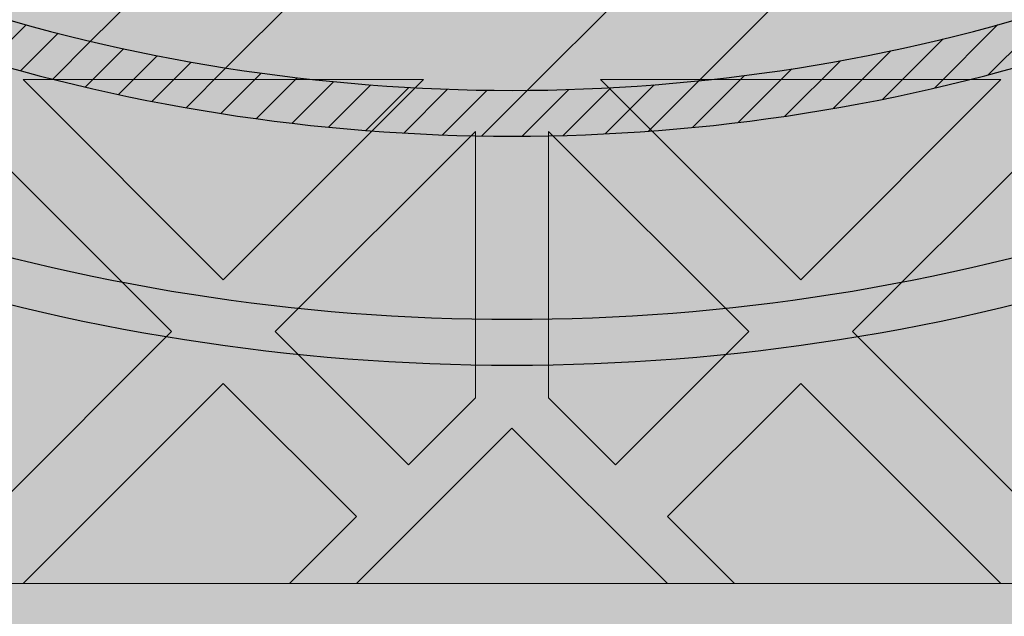
# Model space of a CAD drawing. Units: inches. Extents: x 844 to 2234, y 346 to 1084.
# Tile 10 of 93: x 1121.143 to 1124.57, y 686.542 to 688.619. Entities that reach past the tile are written whole.
import ezdxf

# ---------------------------------------------------------------- set-up
doc = ezdxf.new("R2010")
doc.units = ezdxf.units.IN
doc.header["$MEASUREMENT"] = 0
for name, color, linetype, lineweight in [('A-ANNO-DIMS', 2, 'Continuous', 18), ('furniture', 8, 'Continuous', 18), ('RA-AP-01$0$INT', 35, 'Continuous', 5)]:
    doc.layers.add(name, color=color, linetype=linetype, lineweight=lineweight)
doc.layers.add('RA-AP-01$0$FURN', color=3, linetype='Continuous')
doc.layers.add('RA-AP-01$0$WOOD', color=64, linetype='Continuous')
doc.styles.get("Standard").update_dxf_attribs({"font": 'arial.ttf'})
doc.dimstyles.get("Standard").update_dxf_attribs({"dimtxt": 6, "dimasz": 3, "dimexe": 0.18, "dimexo": 0.0625, "dimgap": 0.09, "dimtad": 0, "dimtih": 1, "dimtoh": 1, "dimdec": 1, "dimzin": 0, "dimdsep": 46, "dimlunit": 3, "dimtxsty": 'Standard', "dimblk": 'ARCHTICK', "dimcen": 0.09, "dimadec": 0, "dimazin": 0, "dimtfac": 1, "dimtdec": 1, "dimtofl": 0, "dimtmove": 0, "dimatfit": 3, "dimfxl": 1, "dimtolj": 1, "dimtzin": 0, "dimarcsym": 0})

# ---------------------------------------------------------------- blocks, each defined once
blk = doc.blocks.new('A$C18D01794')
at = {"layer": 'RA-AP-01$0$INT'}
blk.add_hatch(color=256, dxfattribs=at).paths.add_polyline_path([(4.505206456958071, -6.306712009588038), (5.305206456958072, -6.306712009588038), (5.305206456958072, -7.106712009588038), (5.255206456951893, -7.10671200958804), (5.25520645694868, -6.356712009605972), (4.555206456959269, -6.356712009587461), (4.555206456956052, -7.106712009588038), (4.505206456958073, -7.106712009588038)])
h = blk.add_hatch(color=256, dxfattribs=at)
h.paths.add_polyline_path([(4.585917135068448, -6.356712009588273), (4.614201406330596, -6.356712009589021), (4.668846067270487, -6.411356670531338), (4.723490728212344, -6.356712009591912), (4.771774999457151, -6.35671200959319), (4.826419660396886, -6.411356670535356), (4.862780050090322, -6.374996280843536), (4.844495778842715, -6.356712009595112), (4.862780050090411, -6.356712009595595), (4.905206456960182, -6.399138416468211), (4.947632863832445, -6.356712009597838), (4.965917135079675, -6.356712009598322), (4.947632863831759, -6.374996280845421), (4.983993253523576, -6.411356670538857), (5.038637914464627, -6.356712009600247), (5.08692218571208, -6.356712009601523), (5.141566846649976, -6.411356670541852), (5.196211507589851, -6.356712009604411), (5.224495778822615, -6.356712009605161), (4.905206456953975, -6.676001331473793)])
h.paths.add_polyline_path([(4.895206456956031, -6.637717060225675), (4.895206456958921, -6.528427738347902), (4.840561796018589, -6.583072399285802)], flags=16)
h.paths.add_polyline_path([(4.915206456955638, -6.637717060226121), (4.969851117895509, -6.583072399288678), (4.915206456957609, -6.528427738348344)], flags=16)
h.paths.add_polyline_path([(4.826419660395175, -6.568930263661755), (4.881064321335613, -6.514285602723745), (4.771774999456703, -6.514285602720857)], flags=16)
h.paths.add_polyline_path([(4.983993253519558, -6.568930263665262), (5.038637914460456, -6.514285602726792), (4.929348592581548, -6.514285602724816)], flags=16)
h.paths.add_polyline_path([(4.881064321336025, -6.494285602723742), (4.826419660397532, -6.439640941782821), (4.771774999457062, -6.494285602720859)], flags=16)
h.paths.add_polyline_path([(4.929348592582019, -6.494285602724817), (5.038637914460982, -6.494285602726792), (4.983993253522945, -6.439640941786327)], flags=16)
h.paths.add_polyline_path([(4.895206456960191, -6.480143467100443), (4.895206456962115, -6.407422687715913), (4.876922185715016, -6.389138416467584), (4.840561796021581, -6.425498806159401)], flags=16)
h.paths.add_polyline_path([(4.915206456958487, -6.480143467100889), (4.969851117899527, -6.425498806162279), (4.933490728206909, -6.389138416468043), (4.9152064569598, -6.40742268771434)], flags=16)
h.paths.add_polyline_path([(4.757632863832376, -6.480143467096812), (4.812277524772842, -6.425498806158772), (4.757632863834348, -6.370854145217844)], flags=16)
h.paths.add_polyline_path([(4.737632863832376, -6.480143467096286), (4.737632863834348, -6.370854145217375), (4.682988202893906, -6.425498806155385)], flags=16)
h.paths.add_polyline_path([(5.05278005008503, -6.480143467103376), (5.052780050087917, -6.370854145224413), (4.998135389146995, -6.425498806162908)], flags=16)
h.paths.add_polyline_path([(5.072780050085024, -6.480143467103744), (5.127424711025931, -6.42549880616527), (5.072780050087916, -6.370854145224832)], flags=16)
h.paths.add_polyline_path([(4.935917135072783, -6.706712009592292), (5.255206456948811, -6.387422687716309), (5.255206456948932, -6.415706958964177), (5.200561796010279, -6.470351619902839), (5.255206456949403, -6.524996280841948), (5.25520645694961, -6.5732805520894), (5.200561796009787, -6.627925213029239), (5.236922185702417, -6.664285602721864), (5.255206456949919, -6.646001331474357), (5.255206456949998, -6.664285602721898), (5.212780050078687, -6.706712009592262), (5.25520645695036, -6.749138416463932), (5.255206456950438, -6.767422687711313), (5.236922185702424, -6.749138416463297), (5.200561796009796, -6.785498806155928), (5.255206456950753, -6.840143467096874), (5.25520645695096, -6.888427738341682), (5.200561796010322, -6.943072399282328), (5.255206456951428, -6.997717060223427), (5.255206456951547, -7.026001331471006)])
h.paths.add_polyline_path([(5.042988202883395, -6.785498806155427), (5.097632863823085, -6.840143467095101), (5.097632863822622, -6.730854145216193)], flags=16)
h.paths.add_polyline_path([(5.028846067259663, -6.771356670531693), (5.083490728198774, -6.716712009592573), (4.974201406321001, -6.716712009593042)], flags=16)
h.paths.add_polyline_path([(5.117632863823087, -6.840143467095186), (5.172277524762331, -6.785498806155926), (5.11763286382262, -6.730854145216225)], flags=16)
h.paths.add_polyline_path([(5.08349072819877, -6.696712009593886), (5.028846067259652, -6.642067348654775), (4.974201406320998, -6.696712009593438)], flags=16)
h.paths.add_polyline_path([(5.131774999446817, -6.854285602718917), (5.186419660386065, -6.799640941779662), (5.241064321325782, -6.854285602719365)], flags=17)
h.paths.add_polyline_path([(5.131774999446228, -6.716712009592374), (5.186419660386065, -6.771356670532194), (5.222780050079488, -6.734996280838764), (5.204495778832781, -6.716712009592063)], flags=16)
h.paths.add_polyline_path([(5.097632863822613, -6.682569873970264), (5.097632863823061, -6.573280552091354), (5.042988202883383, -6.627925213031044)], flags=16)
h.paths.add_polyline_path([(5.131774999446899, -6.874285602718915), (5.241064321325809, -6.874285602719364), (5.186419660386591, -6.928930263658598)], flags=17)
h.paths.add_polyline_path([(5.131774999446226, -6.696712009594078), (5.204495778830767, -6.696712009594374), (5.22278005007868, -6.67842773834687), (5.186419660386049, -6.642067348654249)], flags=16)
h.paths.add_polyline_path([(5.11763286382262, -6.682569873970225), (5.17227752476232, -6.627925213030515), (5.117632863823064, -6.573280552091267)], flags=16)
h.paths.add_polyline_path([(5.186419660386069, -6.613783077405491), (5.241064321325754, -6.559138416465795), (5.131774999446791, -6.559138416466263)], flags=16)
h.paths.add_polyline_path([(5.131774999446872, -6.539138416466263), (5.24106432132578, -6.539138416465794), (5.186419660386554, -6.484493755526573)], flags=16)
h.paths.add_polyline_path([(5.255206456951811, -7.08742268770861), (5.255206456951895, -7.106712009588038), (4.555206456956052, -7.106712009588038), (4.555206456956136, -7.087422687708617), (4.905206456953973, -6.737422687710788)])
h.paths.add_polyline_path([(4.983993253513404, -6.8444937555241), (4.92934859257295, -6.899138416462108), (5.03863791445186, -6.899138416465014)], flags=16)
h.paths.add_polyline_path([(4.969851117889988, -6.83035161990006), (4.915206456952556, -6.775706958960171), (4.915206456949648, -6.884996280837944)], flags=16)
h.paths.add_polyline_path([(4.929348592572535, -6.919138416462105), (4.983993253511019, -6.973783077403037), (5.038637914451496, -6.919138416465012)], flags=16)
h.paths.add_polyline_path([(5.052780050074912, -6.93328055208906), (4.998135389134438, -6.987925213027088), (5.052780050072919, -7.042569873968025)], flags=16)
h.paths.add_polyline_path([(5.07278005007491, -6.933280552089588), (5.072780050072918, -7.042569873968497), (5.127424711013374, -6.987925213030498)], flags=16)
h.paths.add_polyline_path([(4.89520645695295, -6.775706958959721), (4.840561796013067, -6.830351619897157), (4.895206456950961, -6.884996280837494)], flags=16)
h.paths.add_polyline_path([(4.915206456948365, -6.933280552085403), (4.915206456946434, -7.006001331471951), (4.933490728192729, -7.024285602719066), (4.969851117886972, -6.987925213026453)], flags=16)
h.paths.add_polyline_path([(4.881064321327021, -6.899138416461022), (4.82641966038902, -6.84449375552057), (4.771774999448108, -6.899138416459029)], flags=16)
h.paths.add_polyline_path([(4.895206456950073, -6.933280552084951), (4.840561796009022, -6.987925213023558), (4.876922185700835, -7.024285602716997), (4.895206456948749, -7.006001331469487)], flags=16)
h.paths.add_polyline_path([(4.983993253510392, -7.0020673486505), (4.947632863816944, -7.038427738342319), (4.965917135064043, -7.05671200959023), (5.038637914448995, -7.056712009591555)], flags=16)
h.paths.add_polyline_path([(4.881064321326543, -6.91913841646102), (4.771774999447578, -6.919138416459031), (4.826419660385607, -6.973783077399508)], flags=16)
h.paths.add_polyline_path([(4.905206456946447, -7.014285602717636), (4.862780050074785, -7.056712009588352), (4.947632863816685, -7.056712009589775)], flags=16)
h.paths.add_polyline_path([(5.14156684663679, -7.002067348654549), (5.086922185696452, -7.056712009592438), (5.196211507574223, -7.056712009594425)], flags=16)
h.paths.add_polyline_path([(4.8264196603837, -7.002067348646972), (4.771774999442643, -7.056712009585575), (4.8444957788276, -7.056712009587508), (4.862780050075511, -7.038427738340416)], flags=16)
h.paths.add_polyline_path([(4.812277524760289, -6.98792521302292), (4.757632863822258, -6.933280552082447), (4.757632863819352, -7.042569873961408)], flags=16)
h.paths.add_polyline_path([(4.73763286382226, -6.933280552082079), (4.682988202881349, -6.987925213020536), (4.737632863819352, -7.04256987396099)], flags=16)
h.paths.add_polyline_path([(4.723490728195188, -7.056712009584289), (4.668846067257299, -7.002067348643949), (4.614201406317417, -7.056712009581383)], flags=16)
h.paths.add_polyline_path([(4.597632863829262, -6.706712009592262), (4.555206456957951, -6.664285602721896), (4.555206456958029, -6.646001331474357), (4.573490728205535, -6.664285602721864), (4.609851117898167, -6.627925213029238), (4.555206456958338, -6.573280552089402), (4.555206456958546, -6.524996280841952), (4.60985111789767, -6.470351619902839), (4.555206456959015, -6.415706958964177), (4.555206456959138, -6.387422687716309), (4.874495778835167, -6.70671200959229), (4.5552064569564, -7.026001331471015), (4.555206456956523, -6.997717060223433), (4.609851117897629, -6.94307239928233), (4.555206456956988, -6.888427738341681), (4.555206456957198, -6.840143467096881), (4.609851117898153, -6.78549880615593), (4.573490728205528, -6.749138416463297), (4.555206456957507, -6.76742268771132), (4.555206456957585, -6.749138416463933)])
h.paths.add_polyline_path([(4.712780050085332, -6.730854145216195), (4.712780050084863, -6.840143467095105), (4.767424711024555, -6.785498806155427)], flags=16)
h.paths.add_polyline_path([(4.726922185709173, -6.716712009592573), (4.781566846648288, -6.771356670531693), (4.836211507586949, -6.716712009593043)], flags=16)
h.paths.add_polyline_path([(4.692780050085327, -6.730854145216225), (4.638135389145619, -6.785498806155928), (4.692780050084865, -6.840143467095185)], flags=16)
h.paths.add_polyline_path([(4.726922185709182, -6.696712009593886), (4.836211507586949, -6.696712009593436), (4.7815668466483, -6.642067348654773)], flags=16)
h.paths.add_polyline_path([(4.678637914461726, -6.71671200959237), (4.605917135075169, -6.716712009592063), (4.587632863828464, -6.734996280838766), (4.623993253521887, -6.771356670532195)], flags=16)
h.paths.add_polyline_path([(4.712780050085336, -6.68256987397026), (4.767424711024568, -6.627925213031042), (4.71278005008489, -6.573280552091352)], flags=16)
h.paths.add_polyline_path([(4.678637914461726, -6.696712009594076), (4.623993253521899, -6.642067348654247), (4.587632863829271, -6.67842773834687), (4.605917135077185, -6.696712009594376)], flags=16)
h.paths.add_polyline_path([(4.692780050085336, -6.682569873970228), (4.692780050084889, -6.573280552091267), (4.638135389145632, -6.627925213030515)], flags=16)
h.paths.add_polyline_path([(4.623993253521885, -6.799640941779662), (4.678637914461131, -6.854285602718915), (4.56934859258217, -6.854285602719365)], flags=17)
h.paths.add_polyline_path([(4.623993253521901, -6.613783077405509), (4.678637914461158, -6.559138416466263), (4.569348592582195, -6.559138416465795)], flags=16)
h.paths.add_polyline_path([(4.678637914461051, -6.874285602718915), (4.623993253521361, -6.928930263658598), (4.569348592582143, -6.874285602719364)], flags=17)
h.paths.add_polyline_path([(4.678637914461076, -6.539138416466263), (4.623993253521399, -6.484493755526573), (4.569348592582167, -6.539138416465796)], flags=16)
h = blk.add_hatch(color=256, dxfattribs=at)
h.paths.add_polyline_path([(4.969851117891331, -6.583072399286455), (4.915206456952669, -6.63771706022511), (4.915206456952222, -6.528427738347337)])
h.paths.add_polyline_path([(4.895206456953064, -6.637717060225108), (4.840561796014413, -6.583072399286448), (4.895206456953533, -6.528427738347335)])
h.paths.add_polyline_path([(4.826419660390684, -6.568930263662714), (4.771774999451003, -6.514285602723024), (4.881064321329913, -6.514285602723489)])
h.paths.add_polyline_path([(4.881064321329884, -6.494285602723492), (4.771774999450921, -6.494285602723024), (4.82641966039018, -6.439640941783778)])
h.paths.add_polyline_path([(4.895206456953734, -6.48014346709988), (4.840561796013912, -6.425498806160046), (4.876922185707337, -6.389138416466622), (4.895206456954043, -6.40742268771333)])
h.paths.add_polyline_path([(4.862780050082808, -6.374996280843689), (4.826419660390178, -6.411356670536314), (4.771774999450351, -6.356712009596481), (4.844495778835303, -6.356712009596181)])
h.paths.add_polyline_path([(4.812277524766446, -6.425498806160041), (4.757632863827191, -6.480143467099289), (4.757632863826741, -6.370854145220329)])
h.paths.add_polyline_path([(4.737632863827191, -6.480143467099214), (4.682988202887508, -6.425498806159518), (4.737632863826743, -6.370854145220299)])
h.paths.add_polyline_path([(4.668846067263777, -6.41135667053579), (4.614201406325123, -6.356712009597128), (4.723490728202894, -6.356712009596675)])
h.paths.add_polyline_path([(4.905206456953846, -6.399138416467422), (4.862780050082654, -6.356712009596229), (4.947632863824561, -6.356712009595756)])
h.paths.add_polyline_path([(4.915206456952028, -6.480143467099882), (4.91520645695173, -6.407422687715346), (4.933490728199234, -6.389138416467428), (4.96985111789186, -6.425498806160055)])
h.paths.add_polyline_path([(5.038637914454841, -6.494285602723048), (4.929348592575874, -6.494285602723497), (4.983993253515593, -6.439640941783787)])
h.paths.add_polyline_path([(4.983993253515065, -6.568930263662725), (4.929348592575849, -6.514285602723495), (5.038637914454755, -6.514285602723045)])
h.paths.add_polyline_path([(5.052780050079843, -6.480143467099317), (4.998135389140595, -6.425498806160058), (5.052780050080309, -6.370854145220356)])
h.paths.add_polyline_path([(4.983993253516868, -6.411356670536324), (4.947632863824241, -6.374996280843694), (4.965917135071747, -6.356712009596188), (5.038637914456701, -6.356712009596504)])
h.paths.add_polyline_path([(5.127424711019533, -6.425498806159557), (5.072780050079843, -6.480143467099239), (5.07278005008031, -6.370854145220326)])
h.paths.add_polyline_path([(5.141566846643269, -6.411356670535829), (5.086922185704154, -6.356712009596707), (5.196211507581929, -6.356712009597176)])
for p, q in [((4.555206456959269, -6.356712009587461), (5.255206456948681, -6.356712009605972)), ((4.771774999458274, -6.356712009594314), (4.826419660396887, -6.411356670535356)), ((4.844495778843225, -6.356712009595625), (4.771774999458274, -6.356712009594314)), ((4.844495778843225, -6.356712009595623), (4.862780050090324, -6.374996280843536)), ((4.947632863832319, -6.356712009597965), (4.862780050090411, -6.356712009595598)), ((4.905206456960184, -6.399138416468211), (4.862780050090411, -6.356712009595598)), ((4.905206456960184, -6.399138416468211), (4.947632863832319, -6.356712009597965)), ((4.965917135079672, -6.356712009598325), (4.947632863831755, -6.374996280845422)), ((4.947632863831757, -6.374996280845422), (4.965917135079625, -6.356712009598373)), ((4.965917135079672, -6.356712009598327), (5.038637914464623, -6.356712009600249)), ((5.038637914464623, -6.356712009600249), (4.983993253523576, -6.411356670538861)), ((4.757632863834348, -6.370854145217847), (4.812277524772842, -6.425498806158774)), ((5.052780050087917, -6.370854145224413), (4.998135389146995, -6.425498806162908)), ((4.826419660396886, -6.411356670535356), (4.862780050090322, -6.374996280843536)), ((4.983993253523578, -6.411356670538861), (4.947632863831757, -6.374996280845422)), ((4.840561796021581, -6.425498806159403), (4.876922185715016, -6.389138416467584)), ((4.895206456959797, -6.407422687713593), (4.876922185715016, -6.389138416467584)), ((4.915206456959793, -6.407422687714346), (4.933490728207705, -6.389138416467247)), ((4.969851117899529, -6.425498806162279), (4.93349072820771, -6.389138416468842)), ((4.895206456962113, -6.407422687715495), (4.895206456960191, -6.480143467100447)), ((4.9152064569598, -6.407422687715939), (4.915206456958485, -6.480143467100891)), ((4.757632863832376, -6.48014346709681), (4.812277524772842, -6.425498806158774)), ((4.895206456960191, -6.480143467100447), (4.840561796021581, -6.425498806159401)), ((4.915206456958485, -6.480143467100891), (4.969851117899529, -6.425498806162277)), ((5.052780050085028, -6.480143467103376), (4.998135389146995, -6.425498806162908)), ((4.771774999457064, -6.494285602720857), (4.826419660397532, -6.439640941782821)), ((4.881064321336027, -6.494285602723744), (4.826419660397532, -6.439640941782821)), ((4.92934859258202, -6.494285602724817), (4.983993253522945, -6.439640941786326)), ((5.038637914460983, -6.494285602726792), (4.983993253522945, -6.439640941786326)), ((4.771774999457064, -6.494285602720857), (4.881064321336027, -6.494285602723744)), ((5.038637914460983, -6.494285602726792), (4.92934859258202, -6.494285602724817))]:
    blk.add_line(p, q, dxfattribs=at)
blk = doc.blocks.new('A$C32926AE1')
at = {"layer": 'RA-AP-01$0$WOOD'}
h = blk.add_hatch(color=256, dxfattribs=at)
h.dxf.hatch_style = 1
h.paths.add_polyline_path([(5.157430609644524, 4.573483066760929, -0.1009492694046607), (5.155401577623758, 4.593365984175333, -0.1842662638101597), (5.172249623284174, 4.638795604568598, 0.2056608120311276), (5.179560981299304, 4.661316324430096, 0.3614336704623542), (5.134352340494423, 4.706524965234944, 0.2056608120311297), (5.111831620632933, 4.699213607219793, -0.1842662638101113), (5.066402000239693, 4.682365561559342, -0.1055311479399994), (5.045656153913092, 4.68467289944697, 0.1567636581983829), (4.763886414745334, 4.684672899446966, -0.1055311479399895), (4.743140568418733, 4.68236556155934, -0.1842662638100833), (4.6977109480255, 4.69921360721979, 0.2056608120302612), (4.675190228164109, 4.706524965234949, 0.3614336704708441), (4.629981587358889, 4.66131632442871, 0.2056608120245944), (4.637292945374126, 4.638795604567974, -0.1842662638101024), (4.654140991034615, 4.59336598417475, -0.1009492694055169), (4.652111959013835, 4.573483066760181, 0.021410119221476), (4.629748025606143, 4.156712009541676, 0.0214101192214795), (4.652111959013809, 3.739940952323101, -0.1009492694059586), (4.654140991034615, 3.720058034908448, -0.1842662638100975), (4.637292945374126, 3.674628414515226, 0.2056608120245705), (4.629981587358889, 3.652107694654492, 0.3614336704708879), (4.675190228164113, 3.606899053848249, 0.2056608120302384), (4.697710948025501, 3.614210411863408, -0.1842662638100995), (4.743140568418738, 3.63105845752386, -0.1055311479402541), (4.763886414745388, 3.628751119636215, 0.1567636581983776), (5.045656153913137, 3.628751119636244, -0.1055311479397538), (5.066402000239692, 3.631058457523857, -0.1842662638101067), (5.111831620632931, 3.614210411863407, 0.2056608120310924), (5.134352340494417, 3.606899053848256, 0.3614336704624001), (5.179560981299307, 3.652107694653103, 0.2056608120311314), (5.172249623284175, 3.6746284145146, -0.1842662638101402), (5.155401577623758, 3.72005803490786, -0.1009492694051366), (5.15743060964455, 3.739940952322354, 0.0214101192215073), (5.179794543052287, 4.156712009541468, 0.0214101192215252)])
h.paths.add_polyline_path([(4.639748609479751, 4.156712009541513, 0.0213537860821624), (4.661970494867118, 3.741887061152232, -0.094075836301374), (4.664143710413708, 3.7196126951003, -0.1824818158568985), (4.644813765429836, 3.668037719127816, 0.2056608120245319), (4.639939526753007, 3.653023905887301, 0.3614336704710246), (4.676106439397173, 3.616856993242342, 0.2056608120302234), (4.691120252638095, 3.621731231919122, -0.1824818158602558), (4.742695228611606, 3.641061176902986, -0.1029891339458722), (4.766991894714349, 3.638256818950944, 0.156709409989566), (5.042550673941472, 3.638256818950105, -0.102989133958497), (5.066847340047078, 3.641061176902949, -0.1824818158594995), (5.118422316020358, 3.621731231919103, 0.2056608120311416), (5.133436129261316, 3.616856993242346, 0.3614336704621468), (5.169603041905217, 3.653023905886178, 0.2056608120310986), (5.164728803228477, 3.668037719127177, -0.1824818158565612), (5.145398858244737, 3.719612695099578, -0.0940758363009313), (5.147572073791232, 3.741887061151398, 0.0213537860822023), (5.169793959178681, 4.156712009541451, 0.0213537860822226), (5.147572073791203, 4.571536957931898, -0.0940758363005034), (5.145398858244737, 4.59381132398362, -0.1824818158565587), (5.164728803228476, 4.645386299956021, 0.2056608120311045), (5.169603041905216, 4.66040011319702, 0.3614336704621845), (5.133436129261313, 4.696567025840856, 0.2056608120310773), (5.118422316020359, 4.691692787164098, -0.182481815859508), (5.066847340047078, 4.67236284218025, -0.1029891339584606), (5.04255067394148, 4.675167200133092, 0.156709409989566), (4.766991894714357, 4.675167200132257, -0.1029891339458842), (4.742695228611611, 4.672362842180213, -0.1824818158602725), (4.691120252638095, 4.691692787164077, 0.2056608120302152), (4.676106439397174, 4.696567025840858, 0.3614336704710363), (4.639939526753005, 4.660400113195899, 0.2056608120245495), (4.644813765429837, 4.645386299955384, -0.1824818158568934), (4.664143710413708, 4.593811323982902, -0.0940758363009187), (4.661970494867149, 4.571536957931074, 0.021353786082177)], flags=16)
h.paths.add_polyline_path([(5.129794543052235, 4.432167055276933, -0.0141661062790638), (5.130152669293814, 4.156927903047693, -0.0141661062790647), (5.129794543052234, 3.881688750818433, -0.0785247771143638), (5.10979738006795, 3.755143611847103, 0.0945969212073497), (5.105408519571111, 3.717898134952927, 0.1043170707844957), (5.116074640131521, 3.670385395016088, 0.1043170707864965), (5.068561900193738, 3.681051515576561, 0.09459692119553), (5.031316423304057, 3.676662655080835, -0.1580239521427272), (4.778226145355827, 3.676662655080367, 0.0945969211986668), (4.740980668464973, 3.681051515576592, 0.1043170707882822), (4.693467928526415, 3.670385395015844, 0.1043170707867916), (4.704134049087309, 3.717898134953662, 0.0945969211972894), (4.69974518859162, 3.755143611844042, -0.0785247771163196), (4.679748025606343, 3.881688750818406, -0.0141661062790663), (4.679389899364763, 4.156927903047693, -0.0141661062790672), (4.679748025606343, 4.432167055276998, -0.0785247771163064), (4.699745188591625, 4.55871219425134, 0.094596921197333), (4.704134049087308, 4.595957671141738, 0.1043170707867205), (4.693467928526416, 4.643470411079523, 0.1043170707882628), (4.740980668464965, 4.632804290518776, 0.0945969211988114), (4.778226145355874, 4.637193151015016, -0.158023952142669), (5.031316423304015, 4.637193151014546, 0.0945969211956361), (5.068561900193736, 4.632804290518806, 0.1043170707864979), (5.11607464013152, 4.643470411079278, 0.1043170707844617), (5.105408519571112, 4.595957671142455, 0.0945969212074597), (5.109797380067959, 4.558712194248236, -0.0785247771143467)], flags=0)
h.paths.add_polyline_path([(5.119794532311105, 4.432259799204851, -0.0142000800617244), (5.120156169157484, 4.156927903047701, -0.0142000800617277), (5.119794532311105, 3.881596006890482, -0.0784894509520253), (5.100273383573699, 3.758192358677797, 0.0940138827242913), (5.095413455884425, 3.717477693979438, 0.0606271852308753), (5.099615656341024, 3.686844378806616, 0.0606271852322524), (5.068982341167493, 3.691046579263239, 0.0940138827010453), (5.028267676478798, 3.686186651576848, -0.1580706864508061), (4.781274892180912, 3.686186651576435, 0.0940138827026903), (4.740560227491556, 3.691046579263279, 0.0606271852339895), (4.709926912317155, 3.686844378806508, 0.0606271852329405), (4.714129112773991, 3.717477693980356, 0.094013882701304), (4.709269185087677, 3.758192358669163, -0.0784894509577193), (4.689748036347473, 3.881596006890469, -0.014200080061729), (4.689386399501094, 4.156927903047709, -0.0142000800617217), (4.689748036347473, 4.432259799204808, -0.078489450957724), (4.709269185087651, 4.555663447426125, 0.0940138827014585), (4.714129112773992, 4.596378112114996, 0.0606271852329731), (4.709926912317154, 4.62701142728886, 0.0606271852340196), (4.74056022749157, 4.622809226832087, 0.0940138827024997), (4.781274892180847, 4.627669154518912, -0.1580706864508359), (5.028267676478777, 4.627669154518526, 0.0940138827010946), (5.068982341167492, 4.622809226832129, 0.060627185232254), (5.099615656341024, 4.627011427288751, 0.0606271852308727), (5.095413455884425, 4.59637811211593, 0.0940138827241088), (5.100273383573675, 4.555663447417647, -0.0784894509520978)], flags=0)
h.paths.add_polyline_path([(5.06978912287499, 4.430218106756144, -0.014241683694547), (5.070173729147532, 4.156927903047672, -0.0142416836945458), (5.06978912287499, 3.883637699339223, -0.0800609523125196), (5.052662118612511, 3.773463122773442, 0.0526421978001116), (5.04590916754064, 3.740550867606997, 0.0526421977992423), (5.012996912374707, 3.73379791653534, -0.1583028414718258), (4.796545656286308, 3.73379791653451, 0.0526421978034211), (4.763633401117837, 3.740550867607021, 0.0526421978018622), (4.756880450045755, 3.773463122774558, -0.0800609523117106), (4.739753445783639, 3.883637699339268, -0.0142416836945435), (4.739368839511098, 4.156927903047671, -0.0142416836945477), (4.739753445783639, 4.430218106756155, -0.0800609523116345), (4.75688045004574, 4.540392683320762, 0.052642197801941), (4.763633401117837, 4.573304938488346, 0.0526421978035071), (4.796545656286361, 4.580057889560873, -0.1583028414717561), (5.012996912374669, 4.580057889560039, 0.0526421977993048), (5.04590916754064, 4.57330493848837, 0.0526421978002057), (5.052662118612529, 4.540392683321868, -0.080060952312477)], flags=0)
h.paths.add_polyline_path([(5.049789715110557, 4.43038092723357, -0.0143097550741839), (5.05018085590259, 4.156927903047715, -0.0143097550741854), (5.049789715110558, 3.883474878861827, -0.0800685599149176), (5.03362098255317, 3.779581877367999, 0.0306258898956367), (5.028241146483733, 3.758218888663947, 0.0306258898977031), (5.006878157778253, 3.75283905259408, -0.1583983521624096), (4.802664410878162, 3.752839052594731, 0.0306258898946014), (4.781301422174808, 3.758218888663924, 0.0306258898967912), (4.775921586105202, 3.779581877368794, -0.080068559914251), (4.759752853548071, 3.883474878861786, -0.0143097550741854), (4.759361712756037, 4.156927903047671, -0.0143097550741854), (4.759752853548071, 4.430380927233557, -0.0800685599142479), (4.775921586105193, 4.534273928726546, 0.0306258898968306), (4.781301422174808, 4.555636917431444, 0.0306258898945754), (4.802664410878143, 4.561016753500631, -0.1583983521624168), (5.006878157778244, 4.561016753501291, 0.0306258898977177), (5.028241146483733, 4.555636917431421, 0.0306258898958182), (5.03362098255321, 4.534273928727244, -0.080068559914796)], flags=0)
h.paths.add_polyline_path([(4.999766070382627, 4.428171244713864, -0.0143443147609634), (5.000198441819402, 4.156927903047689, -0.0143443147609612), (4.999766070382627, 3.885684561381556, -0.0784641635803329), (4.987356730658798, 3.799103304488872, -0.1506053783831347), (4.822185837999821, 3.79910330448882, -0.0784641635803318), (4.809776498276007, 3.885684561381509, -0.014344314760963), (4.809344126839227, 4.156927903047677, -0.0143443147609645), (4.809776498276007, 4.428171244713873, -0.0784641635803192), (4.822185837999822, 4.514752501606549, -0.1506053783831338), (4.987356730658798, 4.514752501606494, -0.078464163580285)], flags=0)
h.paths.add_polyline_path([(4.979755254238824, 4.42764379880488, -0.0143772539198268), (4.980205517789977, 4.156927903047693, -0.0143772539198275), (4.979755254238824, 3.886212007290489, -0.0689242507424422), (4.971183264704897, 3.815276770442801, -0.1296645318904179), (4.838359303953726, 3.815276770442746, -0.0689242507424186), (4.829787314419809, 3.886212007290419, -0.0143772539198292), (4.829337050868653, 4.156927903047653, -0.0143772539198325), (4.829787314419809, 4.427643798804946, -0.0689242507424211), (4.838359303953725, 4.498579035652621, -0.1296645318904187), (4.971183264704897, 4.498579035652565, -0.0689242507424401)], flags=0)
h = blk.add_hatch(color=256, dxfattribs=at)
h.dxf.hatch_style = 1
h.paths.add_polyline_path([(5.145398858244737, 4.59381132398362, -0.1824818158565616), (5.164728803228476, 4.645386299956021, 0.2056608120311045), (5.169603041905216, 4.66040011319702, 0.3614336704621845), (5.133436129261313, 4.696567025840856, 0.2056608120310773), (5.118422316020359, 4.691692787164098, -0.182481815859508), (5.066847340047078, 4.67236284218025, -0.1029891339584606), (5.04255067394148, 4.675167200133092, 0.156709409989566), (4.766991894714357, 4.675167200132257, -0.1029891339458842), (4.742695228611611, 4.672362842180213, -0.1824818158602725), (4.691120252638095, 4.691692787164077, 0.2056608120302152), (4.676106439397174, 4.696567025840858, 0.3614336704710363), (4.639939526753005, 4.660400113195899, 0.2056608120245495), (4.644813765429837, 4.645386299955384, -0.1824818158568934), (4.664143710413708, 4.593811323982902, -0.0940758363009187), (4.661970494867149, 4.571536957931074, 0.0213537860821772), (4.639748609479751, 4.156712009541507, 0.0213537860821625), (4.661970494867119, 3.741887061152226, -0.0940758363013071), (4.664143710413708, 3.719612695100309, -0.1824818158569294), (4.644813765429836, 3.668037719127816, 0.2056608120245319), (4.639939526753007, 3.653023905887301, 0.3614336704710246), (4.676106439397173, 3.616856993242342, 0.2056608120302234), (4.691120252638095, 3.621731231919122, -0.1824818158602558), (4.742695228611606, 3.641061176902986, -0.1029891339458722), (4.766991894714349, 3.638256818950944, 0.156709409989566), (5.042550673941472, 3.638256818950105, -0.102989133958497), (5.066847340047078, 3.641061176902949, -0.1824818158594995), (5.118422316020358, 3.621731231919103, 0.2056608120311416), (5.133436129261316, 3.616856993242346, 0.3614336704621468), (5.169603041905217, 3.653023905886178, 0.2056608120310986), (5.164728803228477, 3.668037719127177, -0.1824818158565612), (5.145398858244737, 3.719612695099578, -0.0940758363009313), (5.147572073791232, 3.741887061151398, 0.0213537860822023), (5.169793959178681, 4.156712009541451, 0.0213537860822226), (5.147572073791203, 4.571536957931898, -0.0940758363004996)])
h.paths.add_polyline_path([(5.109797380067958, 4.55871219424824, -0.0785247771143472), (5.129794543052234, 4.432167055276936, -0.0141661062790644), (5.130152669293814, 4.156927903047685, -0.014166106279066), (5.129794543052234, 3.881688750818401, -0.0785247771143517), (5.109797380067946, 3.755143611847092, 0.0945969212073132), (5.105408519571111, 3.717898134952929, 0.1043170707844995), (5.116074640131521, 3.670385395016088, 0.1043170707864965), (5.068561900193738, 3.681051515576561, 0.09459692119553), (5.031316423304057, 3.676662655080835, -0.1580239521427272), (4.778226145355827, 3.676662655080367, 0.0945969211986668), (4.740980668464973, 3.681051515576592, 0.1043170707882822), (4.693467928526415, 3.670385395015844, 0.1043170707867916), (4.704134049087309, 3.717898134953662, 0.0945969211972894), (4.69974518859162, 3.755143611844042, -0.0785247771163196), (4.679748025606343, 3.881688750818406, -0.0141661062790663), (4.679389899364763, 4.156927903047693, -0.0141661062790672), (4.679748025606343, 4.432167055276998, -0.0785247771163064), (4.699745188591625, 4.55871219425134, 0.094596921197333), (4.704134049087308, 4.595957671141738, 0.1043170707867205), (4.693467928526416, 4.643470411079523, 0.1043170707882628), (4.740980668464965, 4.632804290518776, 0.0945969211988114), (4.778226145355874, 4.637193151015016, -0.158023952142669), (5.031316423304015, 4.637193151014546, 0.0945969211956361), (5.068561900193736, 4.632804290518806, 0.1043170707864979), (5.11607464013152, 4.643470411079278, 0.1043170707844617), (5.105408519571112, 4.595957671142455, 0.0945969212074504)], flags=16)
h.paths.add_polyline_path([(5.100273383573655, 4.55566344741771, -0.0784894509521388), (5.119794532311105, 4.432259799204852, -0.0142000800617252), (5.120156169157484, 4.156927903047686, -0.014200080061726), (5.119794532311105, 3.881596006890502, -0.0784894509520446), (5.100273383573696, 3.758192358677786, 0.0940138827242721), (5.095413455884425, 3.717477693979436, 0.0606271852308692), (5.099615656341024, 3.686844378806616, 0.0606271852322522), (5.068982341167493, 3.691046579263239, 0.0940138827010453), (5.028267676478798, 3.686186651576848, -0.1580706864508061), (4.781274892180912, 3.686186651576435, 0.0940138827026903), (4.740560227491556, 3.691046579263279, 0.0606271852339895), (4.709926912317155, 3.686844378806508, 0.0606271852329405), (4.714129112773991, 3.717477693980356, 0.094013882701304), (4.709269185087677, 3.758192358669163, -0.0784894509577193), (4.689748036347473, 3.881596006890469, -0.014200080061729), (4.689386399501094, 4.156927903047709, -0.0142000800617217), (4.689748036347473, 4.432259799204808, -0.078489450957724), (4.709269185087651, 4.555663447426125, 0.0940138827014585), (4.714129112773992, 4.596378112114996, 0.0606271852329731), (4.709926912317154, 4.62701142728886, 0.0606271852340196), (4.74056022749157, 4.622809226832087, 0.0940138827024997), (4.781274892180847, 4.627669154518912, -0.1580706864508359), (5.028267676478777, 4.627669154518526, 0.0940138827010946), (5.068982341167492, 4.622809226832129, 0.060627185232254), (5.099615656341024, 4.627011427288751, 0.0606271852308727), (5.095413455884425, 4.59637811211593, 0.094013882723957)], flags=0)
h.paths.add_polyline_path([(5.04590916754064, 4.57330493848837, 0.0526421978002057), (5.052662118612529, 4.540392683321868, -0.0800609523124783), (5.06978912287499, 4.430218106756142, -0.0142416836945469), (5.070173729147532, 4.156927903047672, -0.0142416836945458), (5.06978912287499, 3.883637699339223, -0.0800609523125196), (5.052662118612511, 3.773463122773442, 0.0526421978001116), (5.04590916754064, 3.740550867606997, 0.0526421977992423), (5.012996912374707, 3.73379791653534, -0.1583028414718258), (4.796545656286308, 3.73379791653451, 0.0526421978034211), (4.763633401117837, 3.740550867607021, 0.0526421978018622), (4.756880450045755, 3.773463122774558, -0.0800609523117106), (4.739753445783639, 3.883637699339268, -0.0142416836945435), (4.739368839511098, 4.156927903047671, -0.0142416836945477), (4.739753445783639, 4.430218106756155, -0.0800609523116345), (4.75688045004574, 4.540392683320762, 0.052642197801941), (4.763633401117837, 4.573304938488346, 0.0526421978035071), (4.796545656286361, 4.580057889560873, -0.1583028414717561), (5.012996912374669, 4.580057889560039, 0.0526421977993048)], flags=0)
h.paths.add_polyline_path([(5.028241146483733, 4.555636917431422, 0.0306258898956949), (5.033620982553182, 4.534273928727329, -0.0800685599148649), (5.049789715110557, 4.430380927233569, -0.0143097550741839), (5.05018085590259, 4.156927903047715, -0.0143097550741854), (5.049789715110558, 3.883474878861827, -0.0800685599149176), (5.03362098255317, 3.779581877367999, 0.0306258898956367), (5.028241146483733, 3.758218888663947, 0.0306258898977031), (5.006878157778253, 3.75283905259408, -0.1583983521624096), (4.802664410878162, 3.752839052594731, 0.0306258898946014), (4.781301422174808, 3.758218888663924, 0.0306258898967912), (4.775921586105202, 3.779581877368794, -0.080068559914251), (4.759752853548071, 3.883474878861786, -0.0143097550741854), (4.759361712756037, 4.156927903047671, -0.0143097550741854), (4.759752853548071, 4.430380927233557, -0.0800685599142479), (4.775921586105193, 4.534273928726546, 0.0306258898968306), (4.781301422174808, 4.555636917431444, 0.0306258898945754), (4.802664410878143, 4.561016753500631, -0.1583983521624168), (5.006878157778244, 4.561016753501291, 0.0306258898977174)], flags=0)
h.paths.add_polyline_path([(4.987356730658798, 4.514752501606494, -0.0784641635803018), (4.999766070382627, 4.428171244713845, -0.0143443147609637), (5.000198441819402, 4.156927903047665, -0.0143443147609622), (4.999766070382628, 3.885684561381514, -0.0784641635802952), (4.987356730658797, 3.799103304488872, -0.1506053783831338), (4.822185837999821, 3.799103304488819, -0.0784641635803342), (4.809776498276007, 3.885684561381512, -0.0143443147609628), (4.809344126839227, 4.156927903047676, -0.0143443147609646), (4.809776498276007, 4.428171244713873, -0.0784641635803192), (4.822185837999822, 4.514752501606549, -0.1506053783831338)], flags=0)
h.paths.add_polyline_path([(4.971183264704897, 4.498579035652566, -0.0689242507424384), (4.979755254238824, 4.427643798804883, -0.0143772539198276), (4.980205517789977, 4.15692790304768, -0.0143772539198258), (4.979755254238823, 3.88621200729051, -0.0689242507424628), (4.971183264704897, 3.815276770442801, -0.129664531890417), (4.838359303953726, 3.815276770442746, -0.0689242507424186), (4.829787314419809, 3.886212007290419, -0.0143772539198292), (4.829337050868653, 4.156927903047653, -0.0143772539198325), (4.829787314419809, 4.427643798804946, -0.0689242507424211), (4.838359303953725, 4.498579035652621, -0.1296645318904187)], flags=0)
h = blk.add_hatch(dxfattribs=at)
h.set_pattern_fill('ANSI31', color=256, scale=0.05, style=0)
h.set_pattern_definition([(45, (0, 0), (-0.0044194173824159, 0.0044194173824159), [])])
h.paths.add_polyline_path([(5.130152669293814, 4.156927903047704, 0.0141661062790657), (5.129794543052234, 4.432167055276982, 0.0777827904001433), (5.110168979996553, 4.557559993161921, -0.0976515123401879), (5.105408519571111, 4.595957671142454, -0.1043170707844687), (5.116074640131522, 4.64347041107928), (5.099615656341024, 4.627011427288751, 0.0606271852308727), (5.095413455884425, 4.59637811211593, 0.0940138827241088), (5.100273383573675, 4.555663447417647, -0.0784894509520972), (5.119794532311105, 4.432259799204852, -0.0142000800617252), (5.120156169157484, 4.156927903047686, -0.014200080061726), (5.119794532311105, 3.881596006890502, -0.0784894509520446), (5.100273383573696, 3.758192358677786, 0.0940138827242721), (5.095413455884425, 3.717477693979436, 0.0606271852308692), (5.099615656341024, 3.686844378806616), (5.116074640131519, 3.67038539501609, -0.1043170707844594), (5.105408519571112, 3.717898134952912, -0.0976515123401594), (5.11016897999655, 3.756295812933435, 0.0777827904001654), (5.129794543052234, 3.881688750818409, 0.0141661062790665)])
h.paths.add_polyline_path([(5.030164222210597, 3.676291055149937, -0.0976515123472002), (5.068561900193739, 3.681051515576561, -0.1043170707864927), (5.116074640131521, 3.670385395016088), (5.099615656341024, 3.686844378806616, 0.0606271852322522), (5.068982341167493, 3.691046579263239, 0.0940138827010453), (5.028267676478798, 3.686186651576848, -0.1580706864508061), (4.781274892180912, 3.686186651576435, 0.0940138827026903), (4.740560227491556, 3.691046579263279, 0.0606271852339913), (4.709926912317154, 3.686844378806508), (4.693467928526416, 3.670385395015845, -0.1043170707882796), (4.740980668464973, 3.681051515576592, -0.0976515123427246), (4.779378346446416, 3.676291055150394, 0.156512506893803)])
h.paths.add_polyline_path([(4.689748036347473, 3.881596006890472, -0.014200080061729), (4.689386399501094, 4.156927903047712, -0.0142000800617195), (4.689748036347473, 4.432259799204768, -0.078489450957742), (4.709269185087648, 4.555663447426114, 0.0940138827014821), (4.714129112773992, 4.596378112114995, 0.0606271852329748), (4.709926912317154, 4.62701142728886), (4.693467928526414, 4.643470411079524, -0.1043170707867939), (4.704134049087309, 4.595957671141706, -0.09765151234893), (4.699373588660725, 4.557559993157876, 0.0777827903975372), (4.679748025606343, 4.432167055276987, 0.0141661062790675), (4.679389899364763, 4.156927903047675, 0.0141661062790641), (4.679748025606343, 3.88168875081843, 0.0777827903975637), (4.699373588660724, 3.756295812937497, -0.0976515123490278), (4.704134049087308, 3.717898134953629, -0.1043170707867196), (4.693467928526416, 3.670385395015845), (4.709926912317155, 3.686844378806508, 0.0606271852329413), (4.714129112773991, 3.717477693980357, 0.0940138827013084), (4.709269185087676, 3.758192358669166, -0.0784894509577192)])
h.paths.add_polyline_path([(4.779378346446434, 4.63756475094498, -0.0976515123427943), (4.740980668464964, 4.632804290518776, -0.1043170707882609), (4.693467928526416, 4.643470411079523), (4.709926912317154, 4.62701142728886, 0.0606271852340196), (4.74056022749157, 4.622809226832087, 0.0940138827024997), (4.781274892180847, 4.627669154518912, -0.1580706864508359), (5.028267676478777, 4.627669154518526, 0.0940138827010946), (5.068982341167492, 4.622809226832129, 0.060627185232254), (5.099615656341024, 4.627011427288751), (5.116074640131521, 4.643470411079279, -0.1043170707865022), (5.068561900193735, 4.632804290518806, -0.0976515123475899), (5.030164222210446, 4.637564750945479, 0.1565125068936924)])
h = blk.add_hatch(dxfattribs=at)
h.set_pattern_fill('ANSI32', color=256, scale=0.2, style=0)
h.set_pattern_definition([(45, (0, 0), (-0.0530330085889911, 0.0530330085889911), []), (45, (0.035355339, 0), (-0.0530330085889911, 0.0530330085889911), [])])
h.paths.add_polyline_path([(5.119794532311105, 4.432259799204823, 0.0777015974868765), (5.10065834347252, 4.554469821747928, -0.0968902511992216), (5.095413455884425, 4.596378112115931, -0.060627185230871), (5.099615656341024, 4.627011427288751, -0.060627185232254), (5.068982341167492, 4.622809226832129, -0.0968902512198245), (5.027074050790956, 4.628054114423209, 0.1564657949319105), (4.782468517866163, 4.628054114422785, -0.0968902512152247), (4.740560227491555, 4.622809226832088, -0.0606271852339878), (4.709926912317155, 4.627011427288859, -0.0606271852329413), (4.714129112773991, 4.596378112115011, -0.0968902512205338), (4.708884225182929, 4.554469821738175, 0.0777015974804443), (4.689748036347473, 4.43225979920482, 0.0142000800617215), (4.689386399501094, 4.156927903047726, 0.0142000800617273), (4.689748036347473, 3.88159600689052, 0.077701597480541), (4.708884225182985, 3.759385984357019, -0.096890251220082), (4.714129112773992, 3.717477693980371, -0.0606271852329731), (4.709926912317154, 3.686844378806507, -0.060627185233988), (4.740560227491554, 3.691046579263279, -0.0968902512152569), (4.782468517866175, 3.685801691672578, 0.1564657949319236), (5.027074050790988, 3.685801691672169, -0.0968902512197451), (5.068982341167491, 3.691046579263239, -0.0606271852322557), (5.099615656341024, 3.686844378806616, -0.0606271852308727), (5.095413455884425, 3.717477693979438, -0.0968902511991229), (5.100658343472507, 3.7593859843474, 0.0777015974868745), (5.119794532311105, 3.8815960068905, 0.014200080061726), (5.120156169157484, 4.156927903047685, 0.0142000800617238)])
h.paths.add_polyline_path([(5.070173729147531, 4.156927903047684, -0.0142416836945481), (5.06978912287499, 3.883637699339191, -0.0800609523125107), (5.052662118612505, 3.773463122773424, 0.0526421978000811), (5.04590916754064, 3.740550867606997, 0.0526421977993214), (5.012996912374658, 3.733797916535325, -0.1583028414717916), (4.796545656286304, 3.733797916534512, 0.0526421978034138), (4.763633401117837, 3.740550867607021, 0.0526421978018622), (4.756880450045755, 3.773463122774558, -0.0800609523117106), (4.739753445783639, 3.883637699339268, -0.0142416836945435), (4.739368839511098, 4.156927903047671, -0.0142416836945477), (4.739753445783639, 4.430218106756155, -0.0800609523116345), (4.75688045004574, 4.540392683320762, 0.052642197801941), (4.763633401117837, 4.573304938488346, 0.0526421978035071), (4.796545656286361, 4.580057889560873, -0.1583028414717561), (5.012996912374669, 4.580057889560039, 0.0526421977993048), (5.04590916754064, 4.57330493848837, 0.0526421978002057), (5.052662118612529, 4.540392683321868, -0.0800609523124783), (5.06978912287499, 4.430218106756142, -0.0142416836945463)], flags=16)
h.paths.add_polyline_path([(5.050180855902591, 4.156927903047686, -0.0143097550741856), (5.049789715110558, 3.883474878861795, -0.0800685599148126), (5.033620982553202, 3.7795818773681, 0.0306258898957837), (5.028241146483733, 3.758218888663947, 0.0306258898977031), (5.006878157778253, 3.75283905259408, -0.1583983521624096), (4.802664410878162, 3.752839052594731, 0.0306258898946014), (4.781301422174808, 3.758218888663924, 0.0306258898967912), (4.775921586105202, 3.779581877368794, -0.080068559914251), (4.759752853548071, 3.883474878861786, -0.0143097550741854), (4.759361712756037, 4.156927903047671, -0.0143097550741854), (4.759752853548071, 4.430380927233557, -0.0800685599142479), (4.775921586105193, 4.534273928726546, 0.0306258898968306), (4.781301422174808, 4.555636917431444, 0.0306258898945754), (4.802664410878143, 4.561016753500631, -0.1583983521624168), (5.006878157778244, 4.561016753501291, 0.0306258898977177), (5.028241146483733, 4.555636917431421, 0.0306258898958182), (5.03362098255321, 4.534273928727244, -0.0800685599147973), (5.049789715110557, 4.430380927233568, -0.0143097550741854)], flags=0)
h.paths.add_polyline_path([(5.000198441819402, 4.15692790304769, -0.0143443147609622), (4.999766070382627, 3.885684561381539, -0.0784641635803169), (4.987356730658798, 3.799103304488873, -0.1506053783831347), (4.822185837999821, 3.79910330448882, -0.0784641635803318), (4.809776498276007, 3.885684561381509, -0.014344314760963), (4.809344126839227, 4.156927903047677, -0.0143443147609645), (4.809776498276007, 4.428171244713873, -0.0784641635803192), (4.822185837999822, 4.514752501606549, -0.1506053783831338), (4.987356730658798, 4.514752501606494, -0.0784641635803018), (4.999766070382627, 4.428171244713845, -0.0143443147609624)], flags=0)
h.paths.add_polyline_path([(4.980205517789976, 4.156927903047707, -0.0143772539198295), (4.979755254238824, 3.886212007290466, -0.06892425074242), (4.971183264704897, 3.815276770442801, -0.129664531890417), (4.838359303953726, 3.815276770442746, -0.0689242507424186), (4.829787314419809, 3.886212007290419, -0.0143772539198292), (4.829337050868653, 4.156927903047653, -0.0143772539198325), (4.829787314419809, 4.427643798804946, -0.0689242507424211), (4.838359303953725, 4.498579035652621, -0.1296645318904187), (4.971183264704897, 4.498579035652565, -0.0689242507424418), (4.979755254238824, 4.427643798804878, -0.0143772539198259)], flags=0)
for centre, radius, start, end in [((4.904771284329219, 4.067062675376634), 0.4003971832811741, 252.0350753990311, 287.9649246011635), ((4.904771284329219, 4.067062675376636), 0.4103971832811756, 252.0403002450644, 287.9596997551364), ((4.904771284329217, 4.067062675376635), 0.4503971832811742, 252.0623235132636, 287.9376764870612), ((4.904771284329219, 4.067062675376637), 0.4603971832811766, 252.0683908477148, 287.9316091522846)]:
    blk.add_arc(centre, radius, start, end, dxfattribs=at)
blk = doc.blocks.new('A$C5D2F253E')
at = {"layer": 'RA-AP-01$0$FURN', "xscale": -0.7999999999883585, "yscale": 0.7999999999883585, "zscale": 0.8, "rotation": 90}
blk.add_blockref('A$C18D01794', (-5.687757199772477, 4.75791982714071), dxfattribs=at)
at = {"layer": 'RA-AP-01$0$WOOD', "rotation": 270}
blk.add_blockref('A$C32926AE1', (-4.161339601644158, 5.73852594588169), dxfattribs=at)
blk = doc.blocks.new('_ArchTick')
at = {"color": 0, "linetype": 'ByBlock', "const_width": 0.15}
blk.add_lwpolyline([(-0.5, -0.5), (0.5, 0.5)], dxfattribs=at)
blk = doc.blocks.new('*D144')
at = {"layer": 'A-ANNO-DIMS', "color": 0, "lineweight": -2, "transparency": 16777216}
for p, q in [((1096.615948, 439.3732739999999), (1096.615948, 1074.743301)), ((1143.115948, 492.373274), (1143.115948, 1074.743301)), ((1096.615948, 1074.563301), (1102.481950728513, 1074.563301)), ((1143.115948, 1074.563301), (1137.249945271487, 1074.563301))]:
    blk.add_line(p, q, dxfattribs=at)
at = {"layer": 'Defpoints', "color": 0, "transparency": 16777216}
for p in [(1143.115948, 1074.563301), (1143.115948, 492.3107739999999), (1096.615948, 439.3107739999999)]:
    blk.add_point(p, dxfattribs=at)
at = {"layer": 'A-ANNO-DIMS', "color": 0, "lineweight": -2, "transparency": 16777216, "xscale": 3, "yscale": 3, "zscale": 3, "rotation": 180}
blk.add_blockref('_ArchTick', (1096.615948, 1074.563301), dxfattribs=at)
at = {"layer": 'A-ANNO-DIMS', "color": 0, "lineweight": -2, "transparency": 16777216, "xscale": 3, "yscale": 3, "zscale": 3}
blk.add_blockref('_ArchTick', (1143.115948, 1074.563301), dxfattribs=at)
at = {"layer": 'A-ANNO-DIMS', "color": 0, "transparency": 16777216, "insert": (1119.865948, 1074.563301), "char_height": 6, "attachment_point": 5}
blk.add_mtext('\\A1;3\'-10 1/2"', dxfattribs=at)

msp = doc.modelspace()

# ---------------------------------------------------------------- block references
at = {"layer": 'furniture', "xscale": 15.94108302203742, "yscale": 15.94108302203742, "zscale": 15.94108302203742, "rotation": 90}
msp.add_blockref('A$C5D2F253E', (1136.147844094663, 696.2584716700112), dxfattribs=at)

# ---------------------------------------------------------------- dimensions: what is measured, and where the dimension line sits
at = {"layer": 'A-ANNO-DIMS'}
dim = msp.add_linear_dim(base=(1143.115948, 1074.563301), p1=(1096.615948, 439.3107739999999), p2=(1143.115948, 492.3107739999999), dimstyle='Standard', override={"dimdec": 1, "dimlfac": 1, "dimrnd": 0, "dimzin": 1, "dimdsep": 46, "dimlunit": 4, "dimfrac": 2}, dxfattribs=at)
dim.commit()
dim.dimension.update_dxf_attribs({"geometry": '*D144', "text_midpoint": (1119.865948, 1074.563301)})

doc.saveas('drawing.dxf')
